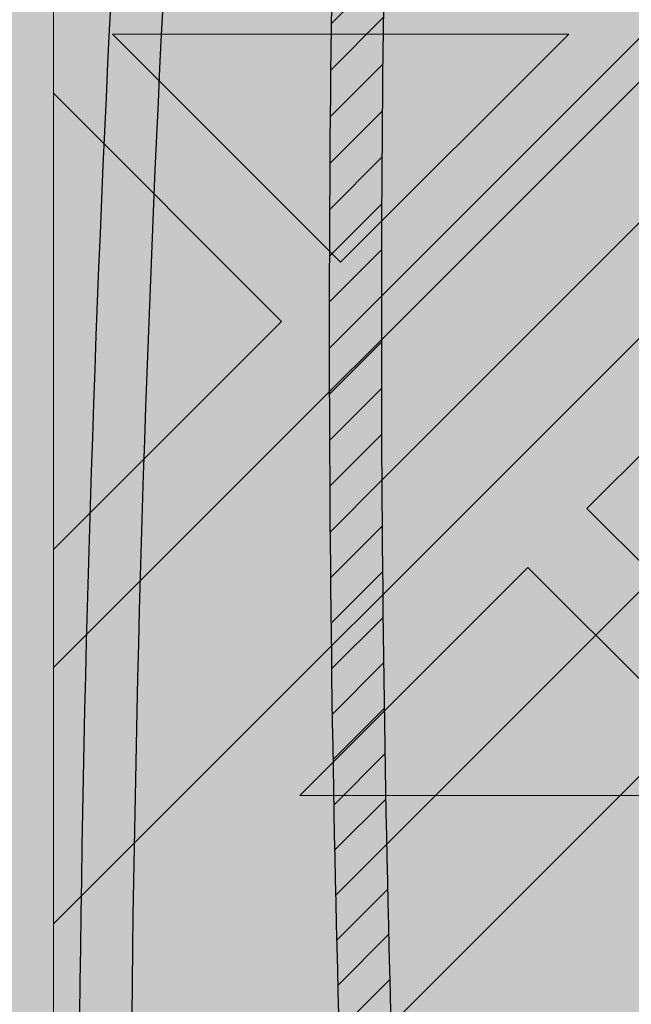
# Model space of a CAD drawing. Units: inches. Extents: x 844 to 2234, y 346 to 1084.
# Tile 15 of 93: x 1118.29 to 1120.159, y 696.22 to 699.229. Entities that reach past the tile are written whole.
import ezdxf

# ---------------------------------------------------------------- set-up
doc = ezdxf.new("R2010")
doc.units = ezdxf.units.IN
doc.header["$MEASUREMENT"] = 0
for name, color, linetype, lineweight in [('A-ANNO-DIMS', 2, 'Continuous', 18), ('furniture', 8, 'Continuous', 18), ('RA-AP-01$0$INT', 35, 'Continuous', 5)]:
    doc.layers.add(name, color=color, linetype=linetype, lineweight=lineweight)
doc.layers.add('RA-AP-01$0$FURN', color=3, linetype='Continuous')
doc.layers.add('RA-AP-01$0$WOOD', color=64, linetype='Continuous')
doc.styles.get("Standard").update_dxf_attribs({"font": 'arial.ttf'})
doc.dimstyles.get("Standard").update_dxf_attribs({"dimtxt": 6, "dimasz": 3, "dimexe": 0.18, "dimexo": 0.0625, "dimgap": 0.09, "dimtad": 0, "dimtih": 1, "dimtoh": 1, "dimdec": 1, "dimzin": 0, "dimdsep": 46, "dimlunit": 3, "dimtxsty": 'Standard', "dimblk": 'ARCHTICK', "dimcen": 0.09, "dimadec": 0, "dimazin": 0, "dimtfac": 1, "dimtdec": 1, "dimtofl": 0, "dimtmove": 0, "dimatfit": 3, "dimfxl": 1, "dimtolj": 1, "dimtzin": 0, "dimarcsym": 0})

# ---------------------------------------------------------------- blocks, each defined once
blk = doc.blocks.new('A$C18D01794')
at = {"layer": 'RA-AP-01$0$INT'}
for points in [[(4.50521, -6.30671), (5.30521, -6.30671), (5.30521, -7.10671), (5.25521, -7.10671), (5.25521, -6.35671), (4.55521, -6.35671), (4.55521, -7.10671), (4.50521, -7.10671)], [(4.50521, -7.90671), (5.30521, -7.90671), (5.30521, -7.10671), (5.25521, -7.10671), (5.25521, -7.85671), (4.55521, -7.85671), (4.55521, -7.10671), (4.50521, -7.10671)]]:
    blk.add_hatch(color=256, dxfattribs=at).paths.add_polyline_path(points)
h = blk.add_hatch(color=256, dxfattribs=at)
h.paths.add_polyline_path([(4.58592, -6.35671), (4.6142, -6.35671), (4.66885, -6.41136), (4.72349, -6.35671), (4.77177, -6.35671), (4.82642, -6.41136), (4.86278, -6.375), (4.8445, -6.35671), (4.86278, -6.35671), (4.90521, -6.39914), (4.94763, -6.35671), (4.96592, -6.35671), (4.94763, -6.375), (4.98399, -6.41136), (5.03864, -6.35671), (5.08692, -6.35671), (5.14157, -6.41136), (5.19621, -6.35671), (5.2245, -6.35671), (4.90521, -6.676)])
h.paths.add_polyline_path([(4.89521, -6.63772), (4.89521, -6.52843), (4.84056, -6.58307)], flags=16)
h.paths.add_polyline_path([(4.91521, -6.63772), (4.96985, -6.58307), (4.91521, -6.52843)], flags=16)
h.paths.add_polyline_path([(4.82642, -6.56893), (4.88106, -6.51429), (4.77177, -6.51429)], flags=16)
h.paths.add_polyline_path([(4.98399, -6.56893), (5.03864, -6.51429), (4.92935, -6.51429)], flags=16)
h.paths.add_polyline_path([(4.88106, -6.49429), (4.82642, -6.43964), (4.77177, -6.49429)], flags=16)
h.paths.add_polyline_path([(4.92935, -6.49429), (5.03864, -6.49429), (4.98399, -6.43964)], flags=16)
h.paths.add_polyline_path([(4.89521, -6.48014), (4.89521, -6.40742), (4.87692, -6.38914), (4.84056, -6.4255)], flags=16)
h.paths.add_polyline_path([(4.91521, -6.48014), (4.96985, -6.4255), (4.93349, -6.38914), (4.91521, -6.40742)], flags=16)
h.paths.add_polyline_path([(4.75763, -6.48014), (4.81228, -6.4255), (4.75763, -6.37085)], flags=16)
h.paths.add_polyline_path([(4.73763, -6.48014), (4.73763, -6.37085), (4.68299, -6.4255)], flags=16)
h.paths.add_polyline_path([(5.05278, -6.48014), (5.05278, -6.37085), (4.99814, -6.4255)], flags=16)
h.paths.add_polyline_path([(5.07278, -6.48014), (5.12742, -6.4255), (5.07278, -6.37085)], flags=16)
h.paths.add_polyline_path([(4.93592, -6.70671), (5.25521, -6.38742), (5.25521, -6.41571), (5.20056, -6.47035), (5.25521, -6.525), (5.25521, -6.57328), (5.20056, -6.62793), (5.23692, -6.66429), (5.25521, -6.646), (5.25521, -6.66429), (5.21278, -6.70671), (5.25521, -6.74914), (5.25521, -6.76742), (5.23692, -6.74914), (5.20056, -6.7855), (5.25521, -6.84014), (5.25521, -6.88843), (5.20056, -6.94307), (5.25521, -6.99772), (5.25521, -7.026)])
h.paths.add_polyline_path([(5.04299, -6.7855), (5.09763, -6.84014), (5.09763, -6.73085)], flags=16)
h.paths.add_polyline_path([(5.02885, -6.77136), (5.08349, -6.71671), (4.9742, -6.71671)], flags=16)
h.paths.add_polyline_path([(5.11763, -6.84014), (5.17228, -6.7855), (5.11763, -6.73085)], flags=16)
h.paths.add_polyline_path([(5.08349, -6.69671), (5.02885, -6.64207), (4.9742, -6.69671)], flags=16)
h.paths.add_polyline_path([(5.13177, -6.85429), (5.18642, -6.79964), (5.24106, -6.85429)], flags=17)
h.paths.add_polyline_path([(5.13177, -6.71671), (5.18642, -6.77136), (5.22278, -6.735), (5.2045, -6.71671)], flags=16)
h.paths.add_polyline_path([(5.09763, -6.68257), (5.09763, -6.57328), (5.04299, -6.62793)], flags=16)
h.paths.add_polyline_path([(5.13177, -6.87429), (5.24106, -6.87429), (5.18642, -6.92893)], flags=17)
h.paths.add_polyline_path([(5.13177, -6.69671), (5.2045, -6.69671), (5.22278, -6.67843), (5.18642, -6.64207)], flags=16)
h.paths.add_polyline_path([(5.11763, -6.68257), (5.17228, -6.62793), (5.11763, -6.57328)], flags=16)
h.paths.add_polyline_path([(5.18642, -6.61378), (5.24106, -6.55914), (5.13177, -6.55914)], flags=16)
h.paths.add_polyline_path([(5.13177, -6.53914), (5.24106, -6.53914), (5.18642, -6.48449)], flags=16)
h.paths.add_polyline_path([(5.25521, -7.08742), (5.25521, -7.10671), (4.55521, -7.10671), (4.55521, -7.08742), (4.90521, -6.73742)])
h.paths.add_polyline_path([(4.98399, -6.84449), (4.92935, -6.89914), (5.03864, -6.89914)], flags=16)
h.paths.add_polyline_path([(4.96985, -6.83035), (4.91521, -6.77571), (4.91521, -6.885)], flags=16)
h.paths.add_polyline_path([(4.92935, -6.91914), (4.98399, -6.97378), (5.03864, -6.91914)], flags=16)
h.paths.add_polyline_path([(5.05278, -6.93328), (4.99814, -6.98793), (5.05278, -7.04257)], flags=16)
h.paths.add_polyline_path([(5.07278, -6.93328), (5.07278, -7.04257), (5.12742, -6.98793)], flags=16)
h.paths.add_polyline_path([(4.89521, -6.77571), (4.84056, -6.83035), (4.89521, -6.885)], flags=16)
h.paths.add_polyline_path([(4.91521, -6.93328), (4.91521, -7.006), (4.93349, -7.02429), (4.96985, -6.98793)], flags=16)
h.paths.add_polyline_path([(4.88106, -6.89914), (4.82642, -6.84449), (4.77177, -6.89914)], flags=16)
h.paths.add_polyline_path([(4.89521, -6.93328), (4.84056, -6.98793), (4.87692, -7.02429), (4.89521, -7.006)], flags=16)
h.paths.add_polyline_path([(4.98399, -7.00207), (4.94763, -7.03843), (4.96592, -7.05671), (5.03864, -7.05671)], flags=16)
h.paths.add_polyline_path([(4.88106, -6.91914), (4.77177, -6.91914), (4.82642, -6.97378)], flags=16)
h.paths.add_polyline_path([(4.90521, -7.01429), (4.86278, -7.05671), (4.94763, -7.05671)], flags=16)
h.paths.add_polyline_path([(5.14157, -7.00207), (5.08692, -7.05671), (5.19621, -7.05671)], flags=16)
h.paths.add_polyline_path([(4.82642, -7.00207), (4.77177, -7.05671), (4.8445, -7.05671), (4.86278, -7.03843)], flags=16)
h.paths.add_polyline_path([(4.81228, -6.98793), (4.75763, -6.93328), (4.75763, -7.04257)], flags=16)
h.paths.add_polyline_path([(4.73763, -6.93328), (4.68299, -6.98793), (4.73763, -7.04257)], flags=16)
h.paths.add_polyline_path([(4.72349, -7.05671), (4.66885, -7.00207), (4.6142, -7.05671)], flags=16)
h.paths.add_polyline_path([(4.59763, -6.70671), (4.55521, -6.66429), (4.55521, -6.646), (4.57349, -6.66429), (4.60985, -6.62793), (4.55521, -6.57328), (4.55521, -6.525), (4.60985, -6.47035), (4.55521, -6.41571), (4.55521, -6.38742), (4.8745, -6.70671), (4.55521, -7.026), (4.55521, -6.99772), (4.60985, -6.94307), (4.55521, -6.88843), (4.55521, -6.84014), (4.60985, -6.7855), (4.57349, -6.74914), (4.55521, -6.76742), (4.55521, -6.74914)])
h.paths.add_polyline_path([(4.71278, -6.73085), (4.71278, -6.84014), (4.76742, -6.7855)], flags=16)
h.paths.add_polyline_path([(4.72692, -6.71671), (4.78157, -6.77136), (4.83621, -6.71671)], flags=16)
h.paths.add_polyline_path([(4.69278, -6.73085), (4.63814, -6.7855), (4.69278, -6.84014)], flags=16)
h.paths.add_polyline_path([(4.72692, -6.69671), (4.83621, -6.69671), (4.78157, -6.64207)], flags=16)
h.paths.add_polyline_path([(4.67864, -6.71671), (4.60592, -6.71671), (4.58763, -6.735), (4.62399, -6.77136)], flags=16)
h.paths.add_polyline_path([(4.71278, -6.68257), (4.76742, -6.62793), (4.71278, -6.57328)], flags=16)
h.paths.add_polyline_path([(4.67864, -6.69671), (4.62399, -6.64207), (4.58763, -6.67843), (4.60592, -6.69671)], flags=16)
h.paths.add_polyline_path([(4.69278, -6.68257), (4.69278, -6.57328), (4.63814, -6.62793)], flags=16)
h.paths.add_polyline_path([(4.62399, -6.79964), (4.67864, -6.85429), (4.56935, -6.85429)], flags=17)
h.paths.add_polyline_path([(4.62399, -6.61378), (4.67864, -6.55914), (4.56935, -6.55914)], flags=16)
h.paths.add_polyline_path([(4.67864, -6.87429), (4.62399, -6.92893), (4.56935, -6.87429)], flags=17)
h.paths.add_polyline_path([(4.67864, -6.53914), (4.62399, -6.48449), (4.56935, -6.53914)], flags=16)
h = blk.add_hatch(color=256, dxfattribs=at)
h.paths.add_polyline_path([(4.58592, -7.85671), (4.6142, -7.85671), (4.66885, -7.80207), (4.72349, -7.85671), (4.77177, -7.85671), (4.82642, -7.80207), (4.86278, -7.83843), (4.8445, -7.85671), (4.86278, -7.85671), (4.90521, -7.81429), (4.94763, -7.85671), (4.96592, -7.85671), (4.94763, -7.83843), (4.98399, -7.80207), (5.03864, -7.85671), (5.08692, -7.85671), (5.14157, -7.80207), (5.19621, -7.85671), (5.2245, -7.85671), (4.90521, -7.53742)])
h.paths.add_polyline_path([(4.89521, -7.57571), (4.89521, -7.685), (4.84056, -7.63035)], flags=16)
h.paths.add_polyline_path([(4.91521, -7.57571), (4.96985, -7.63035), (4.91521, -7.685)], flags=16)
h.paths.add_polyline_path([(4.82642, -7.64449), (4.88106, -7.69914), (4.77177, -7.69914)], flags=16)
h.paths.add_polyline_path([(4.98399, -7.64449), (5.03864, -7.69914), (4.92935, -7.69914)], flags=16)
h.paths.add_polyline_path([(4.88106, -7.71914), (4.82642, -7.77378), (4.77177, -7.71914)], flags=16)
h.paths.add_polyline_path([(4.92935, -7.71914), (5.03864, -7.71914), (4.98399, -7.77378)], flags=16)
h.paths.add_polyline_path([(4.89521, -7.73328), (4.89521, -7.806), (4.87692, -7.82429), (4.84056, -7.78793)], flags=16)
h.paths.add_polyline_path([(4.91521, -7.73328), (4.96985, -7.78793), (4.93349, -7.82429), (4.91521, -7.806)], flags=16)
h.paths.add_polyline_path([(4.75763, -7.73328), (4.81228, -7.78793), (4.75763, -7.84257)], flags=16)
h.paths.add_polyline_path([(4.73763, -7.73328), (4.73763, -7.84257), (4.68299, -7.78793)], flags=16)
h.paths.add_polyline_path([(5.05278, -7.73328), (5.05278, -7.84257), (4.99814, -7.78793)], flags=16)
h.paths.add_polyline_path([(5.07278, -7.73328), (5.12742, -7.78793), (5.07278, -7.84257)], flags=16)
h.paths.add_polyline_path([(4.93592, -7.50671), (5.25521, -7.826), (5.25521, -7.79772), (5.20056, -7.74307), (5.25521, -7.68843), (5.25521, -7.64014), (5.20056, -7.5855), (5.23692, -7.54914), (5.25521, -7.56742), (5.25521, -7.54914), (5.21278, -7.50671), (5.25521, -7.46429), (5.25521, -7.446), (5.23692, -7.46429), (5.20056, -7.42793), (5.25521, -7.37328), (5.25521, -7.325), (5.20056, -7.27035), (5.25521, -7.21571), (5.25521, -7.18742)])
h.paths.add_polyline_path([(5.04299, -7.42793), (5.09763, -7.37328), (5.09763, -7.48257)], flags=16)
h.paths.add_polyline_path([(5.02885, -7.44207), (5.08349, -7.49671), (4.9742, -7.49671)], flags=16)
h.paths.add_polyline_path([(5.11763, -7.37328), (5.17228, -7.42793), (5.11763, -7.48257)], flags=16)
h.paths.add_polyline_path([(5.08349, -7.51671), (5.02885, -7.57136), (4.9742, -7.51671)], flags=16)
h.paths.add_polyline_path([(5.13177, -7.35914), (5.18642, -7.41378), (5.24106, -7.35914)], flags=17)
h.paths.add_polyline_path([(5.13177, -7.49671), (5.18642, -7.44207), (5.22278, -7.47843), (5.2045, -7.49671)], flags=16)
h.paths.add_polyline_path([(5.09763, -7.53085), (5.09763, -7.64014), (5.04299, -7.5855)], flags=16)
h.paths.add_polyline_path([(5.13177, -7.33914), (5.24106, -7.33914), (5.18642, -7.28449)], flags=17)
h.paths.add_polyline_path([(5.13177, -7.51671), (5.2045, -7.51671), (5.22278, -7.535), (5.18642, -7.57136)], flags=16)
h.paths.add_polyline_path([(5.11763, -7.53085), (5.17228, -7.5855), (5.11763, -7.64014)], flags=16)
h.paths.add_polyline_path([(5.18642, -7.59964), (5.24106, -7.65429), (5.13177, -7.65429)], flags=16)
h.paths.add_polyline_path([(5.13177, -7.67429), (5.24106, -7.67429), (5.18642, -7.72893)], flags=16)
h.paths.add_polyline_path([(5.25521, -7.126), (5.25521, -7.10671), (4.55521, -7.10671), (4.55521, -7.126), (4.90521, -7.476)])
h.paths.add_polyline_path([(4.98399, -7.36893), (4.92935, -7.31429), (5.03864, -7.31429)], flags=16)
h.paths.add_polyline_path([(4.96985, -7.38307), (4.91521, -7.43772), (4.91521, -7.32843)], flags=16)
h.paths.add_polyline_path([(4.92935, -7.29429), (4.98399, -7.23964), (5.03864, -7.29429)], flags=16)
h.paths.add_polyline_path([(5.05278, -7.28014), (4.99814, -7.2255), (5.05278, -7.17085)], flags=16)
h.paths.add_polyline_path([(5.07278, -7.28014), (5.07278, -7.17085), (5.12742, -7.2255)], flags=16)
h.paths.add_polyline_path([(4.89521, -7.43772), (4.84056, -7.38307), (4.89521, -7.32843)], flags=16)
h.paths.add_polyline_path([(4.91521, -7.28014), (4.91521, -7.20742), (4.93349, -7.18914), (4.96985, -7.2255)], flags=16)
h.paths.add_polyline_path([(4.88106, -7.31429), (4.82642, -7.36893), (4.77177, -7.31429)], flags=16)
h.paths.add_polyline_path([(4.89521, -7.28014), (4.84056, -7.2255), (4.87692, -7.18914), (4.89521, -7.20742)], flags=16)
h.paths.add_polyline_path([(4.98399, -7.21136), (4.94763, -7.175), (4.96592, -7.15671), (5.03864, -7.15671)], flags=16)
h.paths.add_polyline_path([(4.88106, -7.29429), (4.77177, -7.29429), (4.82642, -7.23964)], flags=16)
h.paths.add_polyline_path([(4.90521, -7.19914), (4.86278, -7.15671), (4.94763, -7.15671)], flags=16)
h.paths.add_polyline_path([(5.14157, -7.21136), (5.08692, -7.15671), (5.19621, -7.15671)], flags=16)
h.paths.add_polyline_path([(4.82642, -7.21136), (4.77177, -7.15671), (4.8445, -7.15671), (4.86278, -7.175)], flags=16)
h.paths.add_polyline_path([(4.81228, -7.2255), (4.75763, -7.28014), (4.75763, -7.17085)], flags=16)
h.paths.add_polyline_path([(4.73763, -7.28014), (4.68299, -7.2255), (4.73763, -7.17085)], flags=16)
h.paths.add_polyline_path([(4.72349, -7.15671), (4.66885, -7.21136), (4.6142, -7.15671)], flags=16)
h.paths.add_polyline_path([(4.59763, -7.50671), (4.55521, -7.54914), (4.55521, -7.56742), (4.57349, -7.54914), (4.60985, -7.5855), (4.55521, -7.64014), (4.55521, -7.68843), (4.60985, -7.74307), (4.55521, -7.79772), (4.55521, -7.826), (4.8745, -7.50671), (4.55521, -7.18742), (4.55521, -7.21571), (4.60985, -7.27035), (4.55521, -7.325), (4.55521, -7.37328), (4.60985, -7.42793), (4.57349, -7.46429), (4.55521, -7.446), (4.55521, -7.46429)])
h.paths.add_polyline_path([(4.71278, -7.48257), (4.71278, -7.37328), (4.76742, -7.42793)], flags=16)
h.paths.add_polyline_path([(4.72692, -7.49671), (4.78157, -7.44207), (4.83621, -7.49671)], flags=16)
h.paths.add_polyline_path([(4.69278, -7.48257), (4.63814, -7.42793), (4.69278, -7.37328)], flags=16)
h.paths.add_polyline_path([(4.72692, -7.51671), (4.83621, -7.51671), (4.78157, -7.57136)], flags=16)
h.paths.add_polyline_path([(4.67864, -7.49671), (4.60592, -7.49671), (4.58763, -7.47843), (4.62399, -7.44207)], flags=16)
h.paths.add_polyline_path([(4.71278, -7.53085), (4.76742, -7.5855), (4.71278, -7.64014)], flags=16)
h.paths.add_polyline_path([(4.67864, -7.51671), (4.62399, -7.57136), (4.58763, -7.535), (4.60592, -7.51671)], flags=16)
h.paths.add_polyline_path([(4.69278, -7.53085), (4.69278, -7.64014), (4.63814, -7.5855)], flags=16)
h.paths.add_polyline_path([(4.62399, -7.41378), (4.67864, -7.35914), (4.56935, -7.35914)], flags=17)
h.paths.add_polyline_path([(4.62399, -7.59964), (4.67864, -7.65429), (4.56935, -7.65429)], flags=16)
h.paths.add_polyline_path([(4.67864, -7.33914), (4.62399, -7.28449), (4.56935, -7.33914)], flags=17)
h.paths.add_polyline_path([(4.67864, -7.67429), (4.62399, -7.72893), (4.56935, -7.67429)], flags=16)
h = blk.add_hatch(color=256, dxfattribs=at)
h.paths.add_polyline_path([(4.90521, -7.53742), (4.8745, -7.50671), (4.55521, -7.826), (4.55521, -7.85671), (4.58592, -7.85671)])
h.paths.add_polyline_path([(4.93592, -7.50671), (4.90521, -7.53742), (5.2245, -7.85671), (5.25521, -7.85671), (5.25521, -7.826)])
h.paths.add_polyline_path([(5.25521, -7.18742), (5.25521, -7.126), (4.90521, -7.476), (4.93592, -7.50671)])
h.paths.add_polyline_path([(4.8745, -7.50671), (4.90521, -7.476), (4.55521, -7.126), (4.55521, -7.18742)])
h = blk.add_hatch(color=256, dxfattribs=at)
h.paths.add_polyline_path([(4.89521, -7.32843), (4.84056, -7.38307), (4.89521, -7.43772)])
h.paths.add_polyline_path([(4.91521, -7.43772), (4.96985, -7.38307), (4.91521, -7.32843)])
h.paths.add_polyline_path([(4.92935, -7.31429), (4.98399, -7.36893), (5.03864, -7.31429)])
h.paths.add_polyline_path([(5.03864, -7.29429), (4.98399, -7.23964), (4.92935, -7.29429)])
h.paths.add_polyline_path([(4.96985, -7.2255), (4.93349, -7.18914), (4.91521, -7.20742), (4.91521, -7.28014)])
h.paths.add_polyline_path([(4.96592, -7.15671), (4.94763, -7.175), (4.98399, -7.21136), (5.03864, -7.15671)])
h.paths.add_polyline_path([(4.99814, -7.2255), (5.05278, -7.28014), (5.05278, -7.17085)])
h.paths.add_polyline_path([(5.07278, -7.28014), (5.12742, -7.2255), (5.07278, -7.17085)])
h.paths.add_polyline_path([(5.19621, -7.15671), (5.08692, -7.15671), (5.14157, -7.21136)])
h.paths.add_polyline_path([(4.86278, -7.15671), (4.90521, -7.19914), (4.94763, -7.15671)])
h.paths.add_polyline_path([(4.89521, -7.28014), (4.89521, -7.20742), (4.87692, -7.18914), (4.84056, -7.2255)])
h.paths.add_polyline_path([(4.82642, -7.23964), (4.77177, -7.29429), (4.88106, -7.29429)])
h.paths.add_polyline_path([(4.77177, -7.31429), (4.82642, -7.36893), (4.88106, -7.31429)])
h.paths.add_polyline_path([(4.75763, -7.28014), (4.81228, -7.2255), (4.75763, -7.17085)])
h.paths.add_polyline_path([(4.86278, -7.175), (4.8445, -7.15671), (4.77177, -7.15671), (4.82642, -7.21136)])
h.paths.add_polyline_path([(4.68299, -7.2255), (4.73763, -7.28014), (4.73763, -7.17085)])
h.paths.add_polyline_path([(4.72349, -7.15671), (4.6142, -7.15671), (4.66885, -7.21136)])
h = blk.add_hatch(color=256, dxfattribs=at)
h.paths.add_polyline_path([(4.78157, -7.44207), (4.83621, -7.49671), (4.72692, -7.49671)])
h.paths.add_polyline_path([(4.83621, -7.51671), (4.78157, -7.57136), (4.72692, -7.51671)])
h.paths.add_polyline_path([(4.76742, -7.5855), (4.71278, -7.64014), (4.71278, -7.53085)])
h.paths.add_polyline_path([(4.69278, -7.53085), (4.69278, -7.64014), (4.63814, -7.5855)])
h.paths.add_polyline_path([(4.67864, -7.51671), (4.62399, -7.57136), (4.58763, -7.535), (4.60592, -7.51671)])
h.paths.add_polyline_path([(4.57349, -7.54914), (4.60985, -7.5855), (4.55521, -7.64014), (4.55521, -7.56742)])
h.paths.add_polyline_path([(4.62399, -7.59964), (4.67864, -7.65429), (4.56935, -7.65429)])
h.paths.add_polyline_path([(4.67864, -7.67429), (4.62399, -7.72893), (4.56935, -7.67429)])
h.paths.add_polyline_path([(4.60985, -7.74307), (4.55521, -7.79772), (4.55521, -7.68843)])
h.paths.add_polyline_path([(4.59763, -7.50671), (4.55521, -7.54914), (4.55521, -7.46429)])
h.paths.add_polyline_path([(4.67864, -7.49671), (4.60592, -7.49671), (4.58763, -7.47843), (4.62399, -7.44207)])
h.paths.add_polyline_path([(4.69278, -7.37328), (4.69278, -7.48257), (4.63814, -7.42793)])
h.paths.add_polyline_path([(4.76742, -7.42793), (4.71278, -7.48257), (4.71278, -7.37328)])
h.paths.add_polyline_path([(4.67864, -7.35914), (4.62399, -7.41378), (4.56935, -7.35914)])
h.paths.add_polyline_path([(4.60985, -7.42793), (4.57349, -7.46429), (4.55521, -7.446), (4.55521, -7.37328)])
h.paths.add_polyline_path([(4.62399, -7.28449), (4.67864, -7.33914), (4.56935, -7.33914)])
h.paths.add_polyline_path([(4.60985, -7.27035), (4.55521, -7.325), (4.55521, -7.21571)])
for p, q in [((4.55521, -7.10671), (4.55521, -6.35671)), ((4.55521, -7.10671), (4.55521, -7.85671)), ((4.90521, -7.476), (4.55521, -7.126)), ((4.72349, -7.15671), (4.6142, -7.15671)), ((4.6142, -7.15671), (4.66885, -7.21136)), ((4.72349, -7.15671), (4.66885, -7.21136)), ((4.73763, -7.17085), (4.68299, -7.2255)), ((4.8745, -7.50671), (4.55521, -7.18742)), ((4.55521, -7.21571), (4.60985, -7.27035)), ((4.55521, -7.325), (4.55521, -7.21571)), ((4.68299, -7.2255), (4.73763, -7.28014)), ((4.55521, -7.325), (4.60985, -7.27035)), ((4.56935, -7.33914), (4.62399, -7.28449)), ((4.62399, -7.28449), (4.67864, -7.33914)), ((4.67864, -7.33914), (4.56935, -7.33914))]:
    blk.add_line(p, q, dxfattribs=at)
blk = doc.blocks.new('A$C32926AE1')
at = {"layer": 'RA-AP-01$0$WOOD'}
h = blk.add_hatch(color=256, dxfattribs=at)
h.dxf.hatch_style = 1
h.paths.add_polyline_path([(5.15743, 4.57348, -0.100949), (5.1554, 4.59337, -0.184266), (5.17225, 4.6388, 0.205661), (5.17956, 4.66132, 0.361434), (5.13435, 4.70652, 0.205661), (5.11183, 4.69921, -0.184266), (5.0664, 4.68237, -0.105531), (5.04566, 4.68467, 0.156764), (4.76389, 4.68467, -0.105531), (4.74314, 4.68237, -0.184266), (4.69771, 4.69921, 0.205661), (4.67519, 4.70652, 0.361434), (4.62998, 4.66132, 0.205661), (4.63729, 4.6388, -0.184266), (4.65414, 4.59337, -0.100949), (4.65211, 4.57348, 0.02141), (4.62975, 4.15671, 0.02141), (4.65211, 3.73994, -0.100949), (4.65414, 3.72006, -0.184266), (4.63729, 3.67463, 0.205661), (4.62998, 3.65211, 0.361434), (4.67519, 3.6069, 0.205661), (4.69771, 3.61421, -0.184266), (4.74314, 3.63106, -0.105531), (4.76389, 3.62875, 0.156764), (5.04566, 3.62875, -0.105531), (5.0664, 3.63106, -0.184266), (5.11183, 3.61421, 0.205661), (5.13435, 3.6069, 0.361434), (5.17956, 3.65211, 0.205661), (5.17225, 3.67463, -0.184266), (5.1554, 3.72006, -0.100949), (5.15743, 3.73994, 0.02141), (5.17979, 4.15671, 0.02141)])
h.paths.add_polyline_path([(4.63975, 4.15671, 0.021354), (4.66197, 3.74189, -0.094076), (4.66414, 3.71961, -0.182482), (4.64481, 3.66804, 0.205661), (4.63994, 3.65302, 0.361434), (4.67611, 3.61686, 0.205661), (4.69112, 3.62173, -0.182482), (4.7427, 3.64106, -0.102989), (4.76699, 3.63826, 0.156709), (5.04255, 3.63826, -0.102989), (5.06685, 3.64106, -0.182482), (5.11842, 3.62173, 0.205661), (5.13344, 3.61686, 0.361434), (5.1696, 3.65302, 0.205661), (5.16473, 3.66804, -0.182482), (5.1454, 3.71961, -0.094076), (5.14757, 3.74189, 0.021354), (5.16979, 4.15671, 0.021354), (5.14757, 4.57154, -0.094076), (5.1454, 4.59381, -0.182482), (5.16473, 4.64539, 0.205661), (5.1696, 4.6604, 0.361434), (5.13344, 4.69657, 0.205661), (5.11842, 4.69169, -0.182482), (5.06685, 4.67236, -0.102989), (5.04255, 4.67517, 0.156709), (4.76699, 4.67517, -0.102989), (4.7427, 4.67236, -0.182482), (4.69112, 4.69169, 0.205661), (4.67611, 4.69657, 0.361434), (4.63994, 4.6604, 0.205661), (4.64481, 4.64539, -0.182482), (4.66414, 4.59381, -0.094076), (4.66197, 4.57154, 0.021354)], flags=16)
h.paths.add_polyline_path([(5.12979, 4.43217, -0.014166), (5.13015, 4.15693, -0.014166), (5.12979, 3.88169, -0.078525), (5.1098, 3.75514, 0.094597), (5.10541, 3.7179, 0.104317), (5.11607, 3.67039, 0.104317), (5.06856, 3.68105, 0.094597), (5.03132, 3.67666, -0.158024), (4.77823, 3.67666, 0.094597), (4.74098, 3.68105, 0.104317), (4.69347, 3.67039, 0.104317), (4.70413, 3.7179, 0.094597), (4.69975, 3.75514, -0.078525), (4.67975, 3.88169, -0.014166), (4.67939, 4.15693, -0.014166), (4.67975, 4.43217, -0.078525), (4.69975, 4.55871, 0.094597), (4.70413, 4.59596, 0.104317), (4.69347, 4.64347, 0.104317), (4.74098, 4.6328, 0.094597), (4.77823, 4.63719, -0.158024), (5.03132, 4.63719, 0.094597), (5.06856, 4.6328, 0.104317), (5.11607, 4.64347, 0.104317), (5.10541, 4.59596, 0.094597), (5.1098, 4.55871, -0.078525)], flags=0)
h.paths.add_polyline_path([(5.11979, 4.43226, -0.0142), (5.12016, 4.15693, -0.0142), (5.11979, 3.8816, -0.078489), (5.10027, 3.75819, 0.094014), (5.09541, 3.71748, 0.060627), (5.09962, 3.68684, 0.060627), (5.06898, 3.69105, 0.094014), (5.02827, 3.68619, -0.158071), (4.78127, 3.68619, 0.094014), (4.74056, 3.69105, 0.060627), (4.70993, 3.68684, 0.060627), (4.71413, 3.71748, 0.094014), (4.70927, 3.75819, -0.078489), (4.68975, 3.8816, -0.0142), (4.68939, 4.15693, -0.0142), (4.68975, 4.43226, -0.078489), (4.70927, 4.55566, 0.094014), (4.71413, 4.59638, 0.060627), (4.70993, 4.62701, 0.060627), (4.74056, 4.62281, 0.094014), (4.78127, 4.62767, -0.158071), (5.02827, 4.62767, 0.094014), (5.06898, 4.62281, 0.060627), (5.09962, 4.62701, 0.060627), (5.09541, 4.59638, 0.094014), (5.10027, 4.55566, -0.078489)], flags=0)
h.paths.add_polyline_path([(5.06979, 4.43022, -0.014242), (5.07017, 4.15693, -0.014242), (5.06979, 3.88364, -0.080061), (5.05266, 3.77346, 0.052642), (5.04591, 3.74055, 0.052642), (5.013, 3.7338, -0.158303), (4.79655, 3.7338, 0.052642), (4.76363, 3.74055, 0.052642), (4.75688, 3.77346, -0.080061), (4.73975, 3.88364, -0.014242), (4.73937, 4.15693, -0.014242), (4.73975, 4.43022, -0.080061), (4.75688, 4.54039, 0.052642), (4.76363, 4.5733, 0.052642), (4.79655, 4.58006, -0.158303), (5.013, 4.58006, 0.052642), (5.04591, 4.5733, 0.052642), (5.05266, 4.54039, -0.080061)], flags=0)
h.paths.add_polyline_path([(5.04979, 4.43038, -0.01431), (5.05018, 4.15693, -0.01431), (5.04979, 3.88347, -0.080069), (5.03362, 3.77958, 0.030626), (5.02824, 3.75822, 0.030626), (5.00688, 3.75284, -0.158398), (4.80266, 3.75284, 0.030626), (4.7813, 3.75822, 0.030626), (4.77592, 3.77958, -0.080069), (4.75975, 3.88347, -0.01431), (4.75936, 4.15693, -0.01431), (4.75975, 4.43038, -0.080069), (4.77592, 4.53427, 0.030626), (4.7813, 4.55564, 0.030626), (4.80266, 4.56102, -0.158398), (5.00688, 4.56102, 0.030626), (5.02824, 4.55564, 0.030626), (5.03362, 4.53427, -0.080069)], flags=0)
h.paths.add_polyline_path([(4.99977, 4.42817, -0.014344), (5.0002, 4.15693, -0.014344), (4.99977, 3.88568, -0.078464), (4.98736, 3.7991, -0.150605), (4.82219, 3.7991, -0.078464), (4.80978, 3.88568, -0.014344), (4.80934, 4.15693, -0.014344), (4.80978, 4.42817, -0.078464), (4.82219, 4.51475, -0.150605), (4.98736, 4.51475, -0.078464)], flags=0)
h.paths.add_polyline_path([(4.97976, 4.42764, -0.014377), (4.98021, 4.15693, -0.014377), (4.97976, 3.88621, -0.068924), (4.97118, 3.81528, -0.129665), (4.83836, 3.81528, -0.068924), (4.82979, 3.88621, -0.014377), (4.82934, 4.15693, -0.014377), (4.82979, 4.42764, -0.068924), (4.83836, 4.49858, -0.129665), (4.97118, 4.49858, -0.068924)], flags=0)
h = blk.add_hatch(color=256, dxfattribs=at)
h.dxf.hatch_style = 1
h.paths.add_polyline_path([(5.1454, 4.59381, -0.182482), (5.16473, 4.64539, 0.205661), (5.1696, 4.6604, 0.361434), (5.13344, 4.69657, 0.205661), (5.11842, 4.69169, -0.182482), (5.06685, 4.67236, -0.102989), (5.04255, 4.67517, 0.156709), (4.76699, 4.67517, -0.102989), (4.7427, 4.67236, -0.182482), (4.69112, 4.69169, 0.205661), (4.67611, 4.69657, 0.361434), (4.63994, 4.6604, 0.205661), (4.64481, 4.64539, -0.182482), (4.66414, 4.59381, -0.094076), (4.66197, 4.57154, 0.021354), (4.63975, 4.15671, 0.021354), (4.66197, 3.74189, -0.094076), (4.66414, 3.71961, -0.182482), (4.64481, 3.66804, 0.205661), (4.63994, 3.65302, 0.361434), (4.67611, 3.61686, 0.205661), (4.69112, 3.62173, -0.182482), (4.7427, 3.64106, -0.102989), (4.76699, 3.63826, 0.156709), (5.04255, 3.63826, -0.102989), (5.06685, 3.64106, -0.182482), (5.11842, 3.62173, 0.205661), (5.13344, 3.61686, 0.361434), (5.1696, 3.65302, 0.205661), (5.16473, 3.66804, -0.182482), (5.1454, 3.71961, -0.094076), (5.14757, 3.74189, 0.021354), (5.16979, 4.15671, 0.021354), (5.14757, 4.57154, -0.094076)])
h.paths.add_polyline_path([(5.1098, 4.55871, -0.078525), (5.12979, 4.43217, -0.014166), (5.13015, 4.15693, -0.014166), (5.12979, 3.88169, -0.078525), (5.1098, 3.75514, 0.094597), (5.10541, 3.7179, 0.104317), (5.11607, 3.67039, 0.104317), (5.06856, 3.68105, 0.094597), (5.03132, 3.67666, -0.158024), (4.77823, 3.67666, 0.094597), (4.74098, 3.68105, 0.104317), (4.69347, 3.67039, 0.104317), (4.70413, 3.7179, 0.094597), (4.69975, 3.75514, -0.078525), (4.67975, 3.88169, -0.014166), (4.67939, 4.15693, -0.014166), (4.67975, 4.43217, -0.078525), (4.69975, 4.55871, 0.094597), (4.70413, 4.59596, 0.104317), (4.69347, 4.64347, 0.104317), (4.74098, 4.6328, 0.094597), (4.77823, 4.63719, -0.158024), (5.03132, 4.63719, 0.094597), (5.06856, 4.6328, 0.104317), (5.11607, 4.64347, 0.104317), (5.10541, 4.59596, 0.094597)], flags=16)
h.paths.add_polyline_path([(5.10027, 4.55566, -0.078489), (5.11979, 4.43226, -0.0142), (5.12016, 4.15693, -0.0142), (5.11979, 3.8816, -0.078489), (5.10027, 3.75819, 0.094014), (5.09541, 3.71748, 0.060627), (5.09962, 3.68684, 0.060627), (5.06898, 3.69105, 0.094014), (5.02827, 3.68619, -0.158071), (4.78127, 3.68619, 0.094014), (4.74056, 3.69105, 0.060627), (4.70993, 3.68684, 0.060627), (4.71413, 3.71748, 0.094014), (4.70927, 3.75819, -0.078489), (4.68975, 3.8816, -0.0142), (4.68939, 4.15693, -0.0142), (4.68975, 4.43226, -0.078489), (4.70927, 4.55566, 0.094014), (4.71413, 4.59638, 0.060627), (4.70993, 4.62701, 0.060627), (4.74056, 4.62281, 0.094014), (4.78127, 4.62767, -0.158071), (5.02827, 4.62767, 0.094014), (5.06898, 4.62281, 0.060627), (5.09962, 4.62701, 0.060627), (5.09541, 4.59638, 0.094014)], flags=0)
h.paths.add_polyline_path([(5.04591, 4.5733, 0.052642), (5.05266, 4.54039, -0.080061), (5.06979, 4.43022, -0.014242), (5.07017, 4.15693, -0.014242), (5.06979, 3.88364, -0.080061), (5.05266, 3.77346, 0.052642), (5.04591, 3.74055, 0.052642), (5.013, 3.7338, -0.158303), (4.79655, 3.7338, 0.052642), (4.76363, 3.74055, 0.052642), (4.75688, 3.77346, -0.080061), (4.73975, 3.88364, -0.014242), (4.73937, 4.15693, -0.014242), (4.73975, 4.43022, -0.080061), (4.75688, 4.54039, 0.052642), (4.76363, 4.5733, 0.052642), (4.79655, 4.58006, -0.158303), (5.013, 4.58006, 0.052642)], flags=0)
h.paths.add_polyline_path([(5.02824, 4.55564, 0.030626), (5.03362, 4.53427, -0.080069), (5.04979, 4.43038, -0.01431), (5.05018, 4.15693, -0.01431), (5.04979, 3.88347, -0.080069), (5.03362, 3.77958, 0.030626), (5.02824, 3.75822, 0.030626), (5.00688, 3.75284, -0.158398), (4.80266, 3.75284, 0.030626), (4.7813, 3.75822, 0.030626), (4.77592, 3.77958, -0.080069), (4.75975, 3.88347, -0.01431), (4.75936, 4.15693, -0.01431), (4.75975, 4.43038, -0.080069), (4.77592, 4.53427, 0.030626), (4.7813, 4.55564, 0.030626), (4.80266, 4.56102, -0.158398), (5.00688, 4.56102, 0.030626)], flags=0)
h.paths.add_polyline_path([(4.98736, 4.51475, -0.078464), (4.99977, 4.42817, -0.014344), (5.0002, 4.15693, -0.014344), (4.99977, 3.88568, -0.078464), (4.98736, 3.7991, -0.150605), (4.82219, 3.7991, -0.078464), (4.80978, 3.88568, -0.014344), (4.80934, 4.15693, -0.014344), (4.80978, 4.42817, -0.078464), (4.82219, 4.51475, -0.150605)], flags=0)
h.paths.add_polyline_path([(4.97118, 4.49858, -0.068924), (4.97976, 4.42764, -0.014377), (4.98021, 4.15693, -0.014377), (4.97976, 3.88621, -0.068924), (4.97118, 3.81528, -0.129665), (4.83836, 3.81528, -0.068924), (4.82979, 3.88621, -0.014377), (4.82934, 4.15693, -0.014377), (4.82979, 4.42764, -0.068924), (4.83836, 4.49858, -0.129665)], flags=0)
h = blk.add_hatch(dxfattribs=at)
h.set_pattern_fill('ANSI31', color=256, scale=0.05, style=0)
h.paths.add_polyline_path([(5.13015, 4.15693, 0.014166), (5.12979, 4.43217, 0.077783), (5.11017, 4.55756, -0.097652), (5.10541, 4.59596, -0.104317), (5.11607, 4.64347), (5.09962, 4.62701, 0.060627), (5.09541, 4.59638, 0.094014), (5.10027, 4.55566, -0.078489), (5.11979, 4.43226, -0.0142), (5.12016, 4.15693, -0.0142), (5.11979, 3.8816, -0.078489), (5.10027, 3.75819, 0.094014), (5.09541, 3.71748, 0.060627), (5.09962, 3.68684), (5.11607, 3.67039, -0.104317), (5.10541, 3.7179, -0.097652), (5.11017, 3.7563, 0.077783), (5.12979, 3.88169, 0.014166)])
h.paths.add_polyline_path([(5.03016, 3.67629, -0.097652), (5.06856, 3.68105, -0.104317), (5.11607, 3.67039), (5.09962, 3.68684, 0.060627), (5.06898, 3.69105, 0.094014), (5.02827, 3.68619, -0.158071), (4.78127, 3.68619, 0.094014), (4.74056, 3.69105, 0.060627), (4.70993, 3.68684), (4.69347, 3.67039, -0.104317), (4.74098, 3.68105, -0.097652), (4.77938, 3.67629, 0.156513)])
h.paths.add_polyline_path([(4.68975, 3.8816, -0.0142), (4.68939, 4.15693, -0.0142), (4.68975, 4.43226, -0.078489), (4.70927, 4.55566, 0.094014), (4.71413, 4.59638, 0.060627), (4.70993, 4.62701), (4.69347, 4.64347, -0.104317), (4.70413, 4.59596, -0.097652), (4.69937, 4.55756, 0.077783), (4.67975, 4.43217, 0.014166), (4.67939, 4.15693, 0.014166), (4.67975, 3.88169, 0.077783), (4.69937, 3.7563, -0.097652), (4.70413, 3.7179, -0.104317), (4.69347, 3.67039), (4.70993, 3.68684, 0.060627), (4.71413, 3.71748, 0.094014), (4.70927, 3.75819, -0.078489)])
h.paths.add_polyline_path([(4.77938, 4.63756, -0.097652), (4.74098, 4.6328, -0.104317), (4.69347, 4.64347), (4.70993, 4.62701, 0.060627), (4.74056, 4.62281, 0.094014), (4.78127, 4.62767, -0.158071), (5.02827, 4.62767, 0.094014), (5.06898, 4.62281, 0.060627), (5.09962, 4.62701), (5.11607, 4.64347, -0.104317), (5.06856, 4.6328, -0.097652), (5.03016, 4.63756, 0.156513)])
h = blk.add_hatch(dxfattribs=at)
h.set_pattern_fill('ANSI32', color=256, scale=0.2, style=0)
h.paths.add_polyline_path([(5.11979, 4.43226, 0.077702), (5.10066, 4.55447, -0.09689), (5.09541, 4.59638, -0.060627), (5.09962, 4.62701, -0.060627), (5.06898, 4.62281, -0.09689), (5.02707, 4.62805, 0.156466), (4.78247, 4.62805, -0.09689), (4.74056, 4.62281, -0.060627), (4.70993, 4.62701, -0.060627), (4.71413, 4.59638, -0.09689), (4.70888, 4.55447, 0.077702), (4.68975, 4.43226, 0.0142), (4.68939, 4.15693, 0.0142), (4.68975, 3.8816, 0.077702), (4.70888, 3.75939, -0.09689), (4.71413, 3.71748, -0.060627), (4.70993, 3.68684, -0.060627), (4.74056, 3.69105, -0.09689), (4.78247, 3.6858, 0.156466), (5.02707, 3.6858, -0.09689), (5.06898, 3.69105, -0.060627), (5.09962, 3.68684, -0.060627), (5.09541, 3.71748, -0.09689), (5.10066, 3.75939, 0.077702), (5.11979, 3.8816, 0.0142), (5.12016, 4.15693, 0.0142)])
h.paths.add_polyline_path([(5.07017, 4.15693, -0.014242), (5.06979, 3.88364, -0.080061), (5.05266, 3.77346, 0.052642), (5.04591, 3.74055, 0.052642), (5.013, 3.7338, -0.158303), (4.79655, 3.7338, 0.052642), (4.76363, 3.74055, 0.052642), (4.75688, 3.77346, -0.080061), (4.73975, 3.88364, -0.014242), (4.73937, 4.15693, -0.014242), (4.73975, 4.43022, -0.080061), (4.75688, 4.54039, 0.052642), (4.76363, 4.5733, 0.052642), (4.79655, 4.58006, -0.158303), (5.013, 4.58006, 0.052642), (5.04591, 4.5733, 0.052642), (5.05266, 4.54039, -0.080061), (5.06979, 4.43022, -0.014242)], flags=16)
h.paths.add_polyline_path([(5.05018, 4.15693, -0.01431), (5.04979, 3.88347, -0.080069), (5.03362, 3.77958, 0.030626), (5.02824, 3.75822, 0.030626), (5.00688, 3.75284, -0.158398), (4.80266, 3.75284, 0.030626), (4.7813, 3.75822, 0.030626), (4.77592, 3.77958, -0.080069), (4.75975, 3.88347, -0.01431), (4.75936, 4.15693, -0.01431), (4.75975, 4.43038, -0.080069), (4.77592, 4.53427, 0.030626), (4.7813, 4.55564, 0.030626), (4.80266, 4.56102, -0.158398), (5.00688, 4.56102, 0.030626), (5.02824, 4.55564, 0.030626), (5.03362, 4.53427, -0.080069), (5.04979, 4.43038, -0.01431)], flags=0)
h.paths.add_polyline_path([(5.0002, 4.15693, -0.014344), (4.99977, 3.88568, -0.078464), (4.98736, 3.7991, -0.150605), (4.82219, 3.7991, -0.078464), (4.80978, 3.88568, -0.014344), (4.80934, 4.15693, -0.014344), (4.80978, 4.42817, -0.078464), (4.82219, 4.51475, -0.150605), (4.98736, 4.51475, -0.078464), (4.99977, 4.42817, -0.014344)], flags=0)
h.paths.add_polyline_path([(4.98021, 4.15693, -0.014377), (4.97976, 3.88621, -0.068924), (4.97118, 3.81528, -0.129665), (4.83836, 3.81528, -0.068924), (4.82979, 3.88621, -0.014377), (4.82934, 4.15693, -0.014377), (4.82979, 4.42764, -0.068924), (4.83836, 4.49858, -0.129665), (4.97118, 4.49858, -0.068924), (4.97976, 4.42764, -0.014377)], flags=0)
for centre, radius, start, end in [((9.50522, 4.10408), 4.87575, 174.47541, 179.3815), ((9.50522, 4.10408), 4.86575, 174.48704, 179.3815), ((9.53595, 4.28823), 4.85833, 178.30224, 181.54738), ((9.53595, 4.28823), 4.84835, 178.3067, 181.55184)]:
    blk.add_arc(centre, radius, start, end, dxfattribs=at)
blk = doc.blocks.new('A$C5D2F253E')
at = {"layer": 'RA-AP-01$0$FURN', "xscale": -0.7999999999883585, "yscale": 0.7999999999883585, "zscale": 0.8, "rotation": 90}
blk.add_blockref('A$C18D01794', (-5.68776, 4.75792), dxfattribs=at)
at = {"layer": 'RA-AP-01$0$WOOD', "rotation": 270}
blk.add_blockref('A$C32926AE1', (-4.16134, 5.73853), dxfattribs=at)
blk = doc.blocks.new('_ArchTick')
at = {"color": 0, "linetype": 'ByBlock', "const_width": 0.15}
blk.add_lwpolyline([(-0.5, -0.5), (0.5, 0.5)], dxfattribs=at)
blk = doc.blocks.new('*D144')
at = {"layer": 'A-ANNO-DIMS', "color": 0, "lineweight": -2, "transparency": 16777216}
for p, q in [((1096.6159, 439.3733), (1096.6159, 1074.7433)), ((1143.1159, 492.3733), (1143.1159, 1074.7433)), ((1096.6159, 1074.5633), (1102.482, 1074.5633)), ((1143.1159, 1074.5633), (1137.2499, 1074.5633))]:
    blk.add_line(p, q, dxfattribs=at)
at = {"layer": 'Defpoints', "color": 0, "transparency": 16777216}
for p in [(1143.1159, 1074.5633), (1143.1159, 492.3108), (1096.6159, 439.3108)]:
    blk.add_point(p, dxfattribs=at)
at = {"layer": 'A-ANNO-DIMS', "color": 0, "lineweight": -2, "transparency": 16777216, "xscale": 3, "yscale": 3, "zscale": 3, "rotation": 180}
blk.add_blockref('_ArchTick', (1096.6159, 1074.5633), dxfattribs=at)
at = {"layer": 'A-ANNO-DIMS', "color": 0, "lineweight": -2, "transparency": 16777216, "xscale": 3, "yscale": 3, "zscale": 3}
blk.add_blockref('_ArchTick', (1143.1159, 1074.5633), dxfattribs=at)
at = {"layer": 'A-ANNO-DIMS', "color": 0, "transparency": 16777216, "insert": (1119.8659, 1074.5633), "char_height": 6, "attachment_point": 5}
blk.add_mtext('\\A1;3\'-10 1/2"', dxfattribs=at)

msp = doc.modelspace()

# ---------------------------------------------------------------- block references
at = {"layer": 'furniture', "xscale": 15.94108302203742, "yscale": 15.94108302203742, "zscale": 15.94108302203742, "rotation": 90}
msp.add_blockref('A$C5D2F253E', (1136.1478, 696.2585), dxfattribs=at)

# ---------------------------------------------------------------- dimensions: what is measured, and where the dimension line sits
at = {"layer": 'A-ANNO-DIMS'}
dim = msp.add_linear_dim(base=(1143.1159, 1074.5633), p1=(1096.6159, 439.3108), p2=(1143.1159, 492.3108), dimstyle='Standard', override={"dimdec": 1, "dimlfac": 1, "dimrnd": 0, "dimzin": 1, "dimdsep": 46, "dimlunit": 4, "dimfrac": 2}, dxfattribs=at)
dim.commit()
dim.dimension.update_dxf_attribs({"geometry": '*D144', "text_midpoint": (1119.8659, 1074.5633)})

doc.saveas('drawing.dxf')
